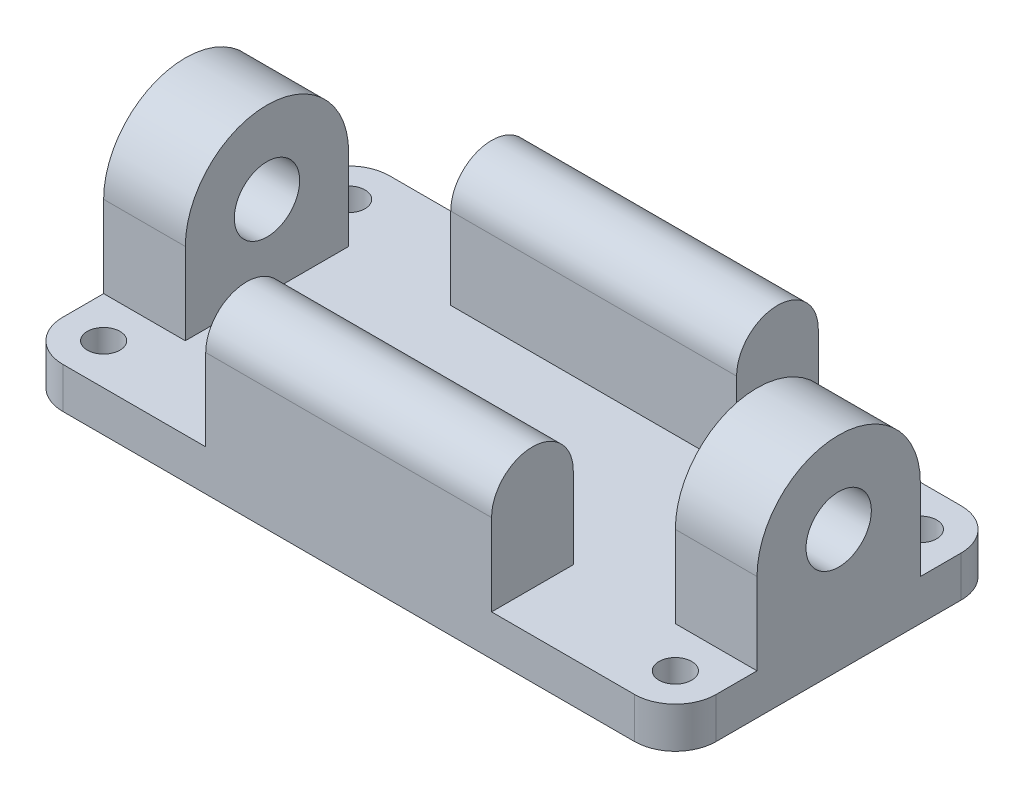
from build123d import *

# Parameters (mm, degrees)
BASE_PLATE_DEPTH        = 5
MOUNTING_HOLES_4_THRU_D = 4
END_LUG_SKETCH_R        = 4
END_LUG_DEPTH           = 10
GUIDE_RAIL_DEPTH        = 17.5


with BuildPart() as part:
    # Base Plate Sketch → Base Plate (new body)
    with BuildSketch(Plane(origin=(0, 0, 0), x_dir=(1, 0, 0), z_dir=(0, 1, 0))):
        with BuildLine():
            Line((-35, -20), (35, -20))
            ThreePointArc((35, -20), (38.535533906, -18.535533906), (40, -15))
            Line((40, -15), (40, 15))
            ThreePointArc((40, 15), (38.535533906, 18.535533906), (35, 20))
            Line((35, 20), (-35, 20))
            ThreePointArc((-35, 20), (-38.535533906, 18.535533906), (-40, 15))
            Line((-40, 15), (-40, -15))
            ThreePointArc((-40, -15), (-38.535533906, -18.535533906), (-35, -20))
        make_face()
    extrude(amount=BASE_PLATE_DEPTH)

    # Mounting Holes Ø4 Thru (through all)
    with Locations(Plane(origin=(-35, 5, -15), x_dir=(0, 0, 1), z_dir=(0, 1, 0))):
        with Locations((0, 0), (0, 70), (30, 70), (30, 0)):
            Hole(MOUNTING_HOLES_4_THRU_D / 2)

    # End Lug Sketch → End Lug (add)
    with BuildSketch(Plane(origin=(40, 0, 0), x_dir=(0, 0, -1), z_dir=(1, 0, 0))):
        with BuildLine():
            Line((-10, 15), (-10, 5))
            Line((-10, 5), (10, 5))
            Line((10, 5), (10, 15))
            ThreePointArc((10, 15), (0, 25), (-10, 15))
        make_face()
        with Locations((0, 15)):
            Circle(END_LUG_SKETCH_R, mode=Mode.SUBTRACT)
    end_lug = extrude(amount=-END_LUG_DEPTH)

    # End Lug Mirror: End Lug across plane
    add(end_lug.mirror(Plane(origin=(0, 0, 0), x_dir=(0, 0, 1), z_dir=(1, 0, 0))))

    # Guide Rail Sketch → Guide Rail (add, symmetric)
    with BuildSketch(Plane(origin=(0, 0, 0), x_dir=(0, 0, -1), z_dir=(1, 0, 0))):
        with BuildLine():
            Line((-20, 5), (-20, 15))
            ThreePointArc((-20, 15), (-15, 20), (-10, 15))
            Line((-10, 15), (-10, 5))
            Line((-10, 5), (-20, 5))
        make_face()
    guide_rail = extrude(amount=GUIDE_RAIL_DEPTH, both=True)

    # Guide Rail Mirror: Guide Rail across plane
    add(guide_rail.mirror(Plane.XY))


solid = part.part
